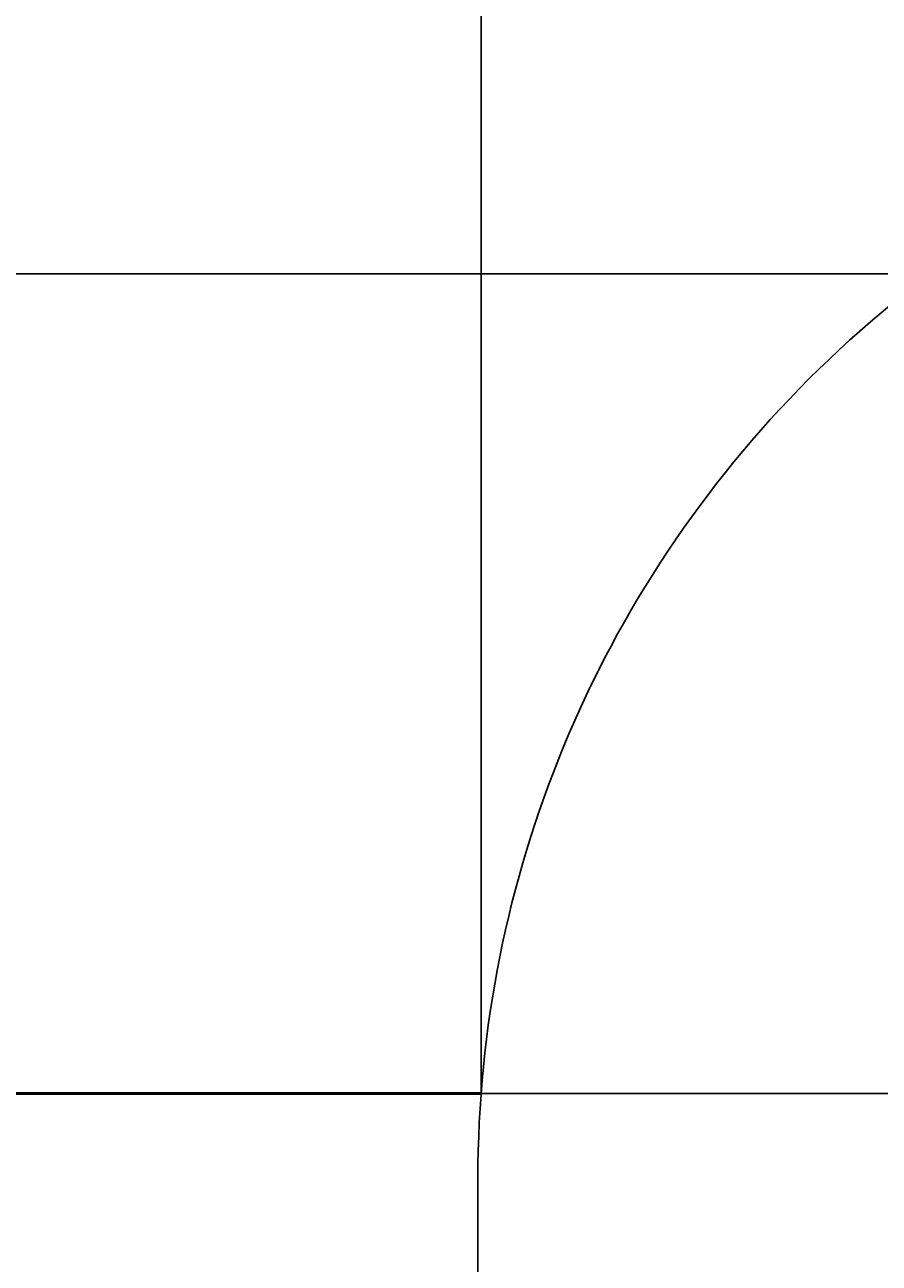
# Model space of a CAD drawing. Units: inches. Extents: x 37 to 824, y -700 to 234.
# Tile 54 of 77: x 234 to 264, y 78 to 122. Entities that reach past the tile are written whole.
import ezdxf

# ---------------------------------------------------------------- set-up
doc = ezdxf.new("R2010")
doc.units = ezdxf.units.IN
doc.header["$MEASUREMENT"] = 0
for name, color, linetype, lineweight in [('A-ANNO-DIMS', 2, 'Continuous', 18), ('A-DOOR', 4, 'Continuous', 25), ('A-WALL', 2, 'Continuous', 50)]:
    doc.layers.add(name, color=color, linetype=linetype, lineweight=lineweight)
doc.styles.get("Standard").update_dxf_attribs({"font": 'arial.ttf'})
doc.dimstyles.get("Standard").update_dxf_attribs({"dimtxt": 0.18, "dimasz": 0.18, "dimexe": 0.18, "dimexo": 0.0625, "dimgap": 0.09, "dimtad": 0, "dimtih": 1, "dimtoh": 1, "dimdec": 1, "dimzin": 0, "dimdsep": 46, "dimlunit": 4, "dimtxsty": 'Standard', "dimcen": 0.09, "dimadec": 0, "dimazin": 0, "dimtfac": 1, "dimtdec": 1, "dimtofl": 0, "dimtmove": 0, "dimatfit": 3, "dimfxl": 1, "dimtolj": 1, "dimtzin": 0, "dimarcsym": 0})

# ---------------------------------------------------------------- blocks, each defined once
blk = doc.blocks.new('*U5')
blk.add_line((40, 0), (40, 6))
blk.add_arc((0, 0), 40, 270, 0)
blk = doc.blocks.new('*D60')
at = {"layer": 'A-ANNO-DIMS', "color": 0, "lineweight": -2, "ltscale": 0.5, "transparency": 16777216}
for p, q in [((419.015, 113.09), (78.159, 113.09)), ((78.339, 112.91), (78.339, 98.772)), ((78.339, 84.27), (78.339, 98.409)), ((419.015, 84.09), (78.159, 84.09))]:
    blk.add_line(p, q, dxfattribs=at)
at = {"layer": 'A-ANNO-DIMS', "color": 0, "ltscale": 0.5, "transparency": 16777216}
for points in [[(78.309, 112.91), (78.369, 112.91), (78.339, 113.09)], [(78.309, 84.27), (78.369, 84.27), (78.339, 84.09)]]:
    blk.add_solid(points, dxfattribs=at)
at = {"layer": 'Defpoints', "color": 0, "ltscale": 0.5, "transparency": 16777216}
for p in [(78.339, 113.09), (419.077, 113.09), (419.077, 84.09)]:
    blk.add_point(p, dxfattribs=at)
at = {"layer": 'A-ANNO-DIMS', "color": 0, "ltscale": 0.5, "transparency": 16777216, "insert": (78.339, 98.59), "char_height": 0.18, "attachment_point": 5}
blk.add_mtext('\\A1;2\'-5"', dxfattribs=at)
blk = doc.blocks.new('*D72')
at = {"layer": 'A-ANNO-DIMS', "color": 0, "lineweight": -2, "ltscale": 0.5, "transparency": 16777216}
for p, q in [((170.077, 84.153), (170.077, 234.17)), ((170.257, 233.99), (209.804, 233.99)), ((250.01, 233.99), (210.463, 233.99)), ((250.19, 84.153), (250.19, 234.17))]:
    blk.add_line(p, q, dxfattribs=at)
at = {"layer": 'A-ANNO-DIMS', "color": 0, "ltscale": 0.5, "transparency": 16777216}
for points in [[(170.257, 234.02), (170.257, 233.96), (170.077, 233.99)], [(250.01, 234.02), (250.01, 233.96), (250.19, 233.99)]]:
    blk.add_solid(points, dxfattribs=at)
at = {"layer": 'Defpoints', "color": 0, "ltscale": 0.5, "transparency": 16777216}
for p in [(250.19, 233.99), (170.077, 84.09), (250.19, 84.09)]:
    blk.add_point(p, dxfattribs=at)
at = {"layer": 'A-ANNO-DIMS', "color": 0, "ltscale": 0.5, "transparency": 16777216, "insert": (210.133, 233.99), "char_height": 0.18, "attachment_point": 5}
blk.add_mtext('\\A1;6\'-8"', dxfattribs=at)
blk = doc.blocks.new('*D73')
at = {"layer": 'A-ANNO-DIMS', "color": 0, "lineweight": -2, "ltscale": 0.5, "transparency": 16777216}
for p, q in [((250.19, 84.153), (250.19, 234.17)), ((250.37, 233.99), (269.804, 233.99)), ((289.897, 233.99), (270.463, 233.99)), ((290.077, 81.153), (290.077, 234.17))]:
    blk.add_line(p, q, dxfattribs=at)
at = {"layer": 'A-ANNO-DIMS', "color": 0, "ltscale": 0.5, "transparency": 16777216}
for points in [[(250.37, 234.02), (250.37, 233.96), (250.19, 233.99)], [(289.897, 234.02), (289.897, 233.96), (290.077, 233.99)]]:
    blk.add_solid(points, dxfattribs=at)
at = {"layer": 'Defpoints', "color": 0, "ltscale": 0.5, "transparency": 16777216}
for p in [(290.077, 233.99), (250.19, 84.09), (290.077, 81.09)]:
    blk.add_point(p, dxfattribs=at)
at = {"layer": 'A-ANNO-DIMS', "color": 0, "ltscale": 0.5, "transparency": 16777216, "insert": (270.133, 233.99), "char_height": 0.18, "attachment_point": 5}
blk.add_mtext('\\A1;3\'-4"', dxfattribs=at)
blk = doc.blocks.new('*D87')
at = {"layer": 'A-ANNO-DIMS', "color": 0, "lineweight": -2, "ltscale": 0.5, "transparency": 16777216}
for p, q in [((216.077, -356.847), (216.077, 234.17)), ((216.257, 233.99), (255.747, 233.99)), ((295.897, 233.99), (256.407, 233.99)), ((296.077, -356.847), (296.077, 234.17))]:
    blk.add_line(p, q, dxfattribs=at)
at = {"layer": 'A-ANNO-DIMS', "color": 0, "ltscale": 0.5, "transparency": 16777216}
for points in [[(216.257, 234.02), (216.257, 233.96), (216.077, 233.99)], [(295.897, 234.02), (295.897, 233.96), (296.077, 233.99)]]:
    blk.add_solid(points, dxfattribs=at)
at = {"layer": 'Defpoints', "color": 0, "ltscale": 0.5, "transparency": 16777216}
for p in [(296.077, 233.99), (216.077, -356.91), (296.077, -356.91)]:
    blk.add_point(p, dxfattribs=at)
at = {"layer": 'A-ANNO-DIMS', "color": 0, "ltscale": 0.5, "transparency": 16777216, "insert": (256.077, 233.99), "char_height": 0.18, "attachment_point": 5}
blk.add_mtext('\\A1;6\'-8"', dxfattribs=at)

msp = doc.modelspace()

# ---------------------------------------------------------------- linework, layer by layer
at = {"layer": 'A-WALL'}
msp.add_line((250.19, 84.09), (170.077, 84.09), dxfattribs=at)

# ---------------------------------------------------------------- block references
at = {"layer": 'A-DOOR', "rotation": 180}
msp.add_blockref('*U5', (290.077, 81.09), dxfattribs=at)

# ---------------------------------------------------------------- dimensions: what is measured, and where the dimension line sits
at = {"layer": 'A-ANNO-DIMS', "ltscale": 0.5}
for base, p1, p2, picture, middle in [((250.19, 233.99), (170.077, 84.09), (250.19, 84.09), '*D72', (210.133, 233.99)), ((296.077, 233.99), (216.077, -356.91), (296.077, -356.91), '*D87', (256.077, 233.99)), ((290.077, 233.99), (250.19, 84.09), (290.077, 81.09), '*D73', (270.133, 233.99))]:
    dim = msp.add_linear_dim(base=base, p1=p1, p2=p2, dimstyle='Standard', override={"dimdec": 1, "dimlfac": 1, "dimrnd": 0, "dimzin": 1, "dimdsep": 46, "dimlunit": 4, "dimfrac": 2}, dxfattribs=at)
    dim.commit()
    dim.dimension.update_dxf_attribs({"geometry": picture, "text_midpoint": middle})
dim = msp.add_linear_dim(base=(78.339, 113.09), p1=(419.077, 84.09), p2=(419.077, 113.09), angle=90, dimstyle='Standard', override={"dimdec": 1, "dimlfac": 1, "dimrnd": 0, "dimzin": 1, "dimdsep": 46, "dimlunit": 4, "dimfrac": 2}, dxfattribs=at)
dim.commit()
dim.dimension.update_dxf_attribs({"geometry": '*D60', "text_midpoint": (78.339, 98.59)})

doc.saveas('drawing.dxf')
